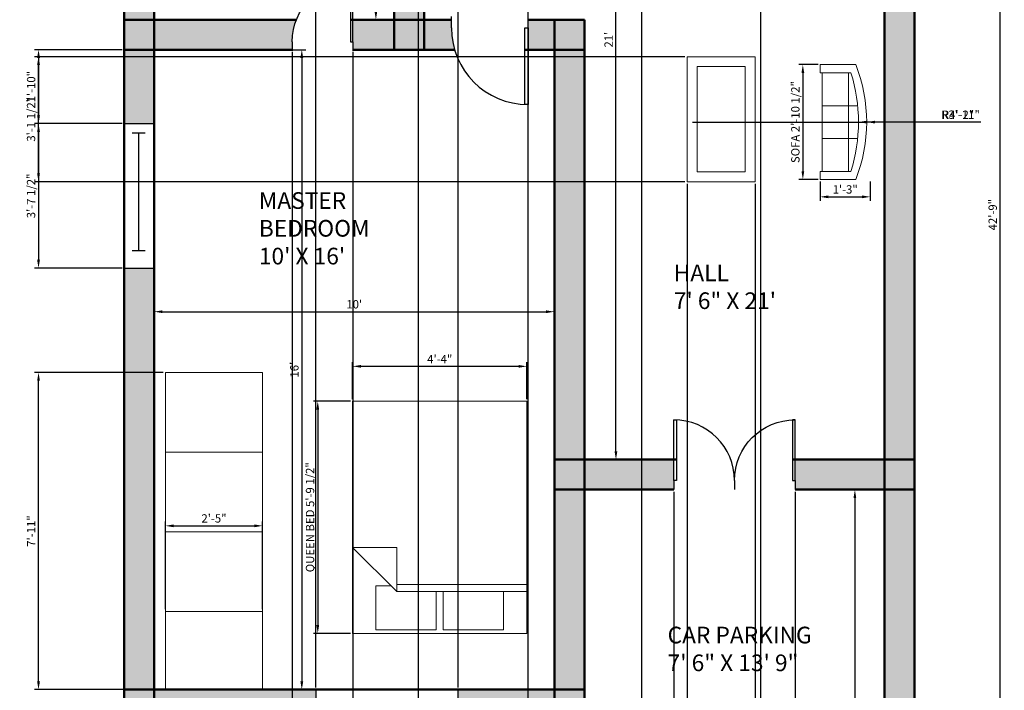
# Model space of a CAD drawing. Units: millimetres. Extents: x 2877 to 3173, y 802 to 1374.
# Tile 2 of 5: x 2877 to 3173, y 943 to 1144. Entities that reach past the tile are written whole.
import ezdxf

# ---------------------------------------------------------------- set-up
doc = ezdxf.new("R2010")
doc.units = ezdxf.units.MM
for name, color, linetype, lineweight in [('A-AREA-IDEN', 150, 'Continuous', 25), ('A-WALL-PATT', 3, 'Continuous', 13), ('dimensions', 140, 'Continuous', 18), ('doors', 10, 'Continuous', 25), ('furniture', 70, 'Continuous', 18), ('walls', 50, 'Continuous', 50), ('windows', 190, 'Continuous', 25)]:
    doc.layers.add(name, color=color, linetype=linetype, lineweight=lineweight)
doc.styles.get("Standard").update_dxf_attribs({"font": 'arial.ttf'})
doc.dimstyles.new('ISO-25', dxfattribs={"dimtxt": 2.5, "dimasz": 2.5, "dimexe": 1.25, "dimexo": 0.625, "dimtad": 1, "dimdec": 0, "dimlunit": 3, "dimtxsty": 'Standard', "dimcen": 2.5, "dimadec": 0, "dimazin": 0, "dimtfac": 1, "dimtdec": 0, "dimtmove": 0, "dimatfit": 3, "dimfxl": 1, "dimarcsym": 0})

# ---------------------------------------------------------------- blocks, each defined once
blk = doc.blocks.new('*U2')
for p, q in [((0, 0), (0, -6)), ((40, 0), (40, -6))]:
    blk.add_line(p, q)
blk.add_lwpolyline([(0, 0), (0, 40), (1.75, 40), (1.75, 0)], close=True)
blk.add_arc((0, 0), 40, 0, 90)
blk = doc.blocks.new('*U4')
for p, q in [((0, 4), (0, 0)), ((36, 4), (36, 0)), ((0, 2), (36, 2))]:
    blk.add_line(p, q)
blk = doc.blocks.new('Bed - Queen')
for p, q in [((0, -80.00003), (0, 0)), ((0, 0), (59.99999, 0)), ((59.99999, 0), (59.99999, -80.00003)), ((7.99999, -1.2), (28.79998, -1.2)), ((7.99999, -14.4), (7.99999, -1.2)), ((28.79998, -1.2), (28.79998, -14.4)), ((31.19999, -1.2), (51.99999, -1.2)), ((31.19999, -14.4), (31.19999, -1.2)), ((51.99999, -1.2), (51.99999, -16.4)), ((0, -14.4), (44.8, -14.4)), ((44.8, -16.8), (0, -16.8)), ((59.99999, -29.6), (44.8, -14.4)), ((44.8, -14.4), (44.8, -29.6)), ((51.99999, -16.4), (46.79936, -16.4)), ((44.8, -29.6), (59.99999, -29.6)), ((59.99999, -80.00003), (0, -80.00003))]:
    blk.add_line(p, q)
blk = doc.blocks.new('Sofa - Roundback 7 ft.')
for p, q in [((-12.00002, -32.4421), (-12.00003, -6.5971)), ((11.99997, -32.4421), (11.99998, -6.5971)), ((-36.000027, -34), (-36.000027, -11.4696)), ((-35.999844, -13.3819), (35.9998, -13.3819)), ((35.99998, -34), (35.99998, -11.4696)), ((-36.000027, -32.4421), (35.99998, -32.4421))]:
    blk.add_line(p, q)
for points in [[(-36.000027, -34), (-42.000027, -34), (-42.000027, -8)], [(41.99998, -8), (41.99998, -34), (35.99998, -34)]]:
    blk.add_lwpolyline(points)
for centre, radius, start, end in [((0, -114.25), 114.25, 68.43141, 111.5686), ((-0.00001, -127.1968), 121.1968, 72.72033, 107.2797)]:
    blk.add_arc(centre, radius, start, end)
blk = doc.blocks.new('*D15')
at = {"layer": 'Defpoints', "color": 0, "transparency": 16777216}
for p in [(3056.09, 1264.28), (3061, 1264.28), (3061, 1012.28)]:
    blk.add_point(p, dxfattribs=at)
at = {"layer": 'dimensions', "color": 0, "lineweight": -2, "transparency": 16777216}
for p, q in [((3060.38, 1264.28), (3054.84, 1264.28)), ((3056.09, 1014.78), (3056.09, 1261.78)), ((3060.38, 1012.28), (3054.84, 1012.28))]:
    blk.add_line(p, q, dxfattribs=at)
at = {"layer": 'dimensions', "color": 0, "transparency": 16777216}
for points in [[(3055.67, 1261.78), (3056.5, 1261.78), (3056.09, 1264.28)], [(3055.67, 1014.78), (3056.5, 1014.78), (3056.09, 1012.28)]]:
    blk.add_solid(points, dxfattribs=at)
at = {"layer": 'dimensions', "color": 0, "transparency": 16777216, "insert": (3054.21, 1138.28), "char_height": 2.5, "attachment_point": 5, "rotation": 90}
blk.add_mtext("21'", dxfattribs=at)
blk = doc.blocks.new('*D16')
at = {"layer": 'Defpoints', "color": 0, "transparency": 16777216}
for p in [(2984.11, 1204.28), (2984.11, 1144.28), (2984.11, 1144.28)]:
    blk.add_point(p, dxfattribs=at)
at = {"layer": 'dimensions', "color": 0, "lineweight": -2, "transparency": 16777216}
for p, q in [((2984.11, 1201.78), (2984.11, 1146.78)), ((2984.74, 1204.28), (2985.36, 1204.28)), ((2984.74, 1144.28), (2985.36, 1144.28))]:
    blk.add_line(p, q, dxfattribs=at)
at = {"layer": 'dimensions', "color": 0, "transparency": 16777216}
for points in [[(2983.69, 1201.78), (2984.53, 1201.78), (2984.11, 1204.28)], [(2983.69, 1146.78), (2984.53, 1146.78), (2984.11, 1144.28)]]:
    blk.add_solid(points, dxfattribs=at)
at = {"layer": 'dimensions', "color": 0, "transparency": 16777216, "insert": (2982.21, 1174.28), "char_height": 2.5, "attachment_point": 5, "rotation": 90}
blk.add_mtext("5'", dxfattribs=at)
blk = doc.blocks.new('*D18')
at = {"layer": 'Defpoints', "color": 0, "transparency": 16777216}
for p in [(2917.62, 1056.67), (3037.62, 1056.67), (3037.62, 1056.67)]:
    blk.add_point(p, dxfattribs=at)
at = {"layer": 'dimensions', "color": 0, "lineweight": -2, "transparency": 16777216}
for p, q in [((2917.62, 1057.29), (2917.62, 1057.92)), ((3037.62, 1057.29), (3037.62, 1057.92)), ((2920.12, 1056.67), (3035.12, 1056.67))]:
    blk.add_line(p, q, dxfattribs=at)
at = {"layer": 'dimensions', "color": 0, "transparency": 16777216}
for points in [[(2920.12, 1057.08), (2920.12, 1056.25), (2917.62, 1056.67)], [(3035.12, 1057.08), (3035.12, 1056.25), (3037.62, 1056.67)]]:
    blk.add_solid(points, dxfattribs=at)
at = {"layer": 'dimensions', "color": 0, "transparency": 16777216, "insert": (2977.62, 1058.57), "char_height": 2.5, "attachment_point": 5}
blk.add_mtext("10'", dxfattribs=at)
blk = doc.blocks.new('*D19')
at = {"layer": 'Defpoints', "color": 0, "transparency": 16777216}
for p in [(2948.77, 1135.28), (2950.14, 943.28), (2961.9, 943.28)]:
    blk.add_point(p, dxfattribs=at)
at = {"layer": 'dimensions', "color": 0, "lineweight": -2, "transparency": 16777216}
for p, q in [((2949.39, 1135.28), (2963.15, 1135.28)), ((2961.9, 1132.78), (2961.9, 945.78)), ((2950.76, 943.28), (2963.15, 943.28))]:
    blk.add_line(p, q, dxfattribs=at)
at = {"layer": 'dimensions', "color": 0, "transparency": 16777216}
for points in [[(2961.48, 1132.78), (2962.32, 1132.78), (2961.9, 1135.28)], [(2961.48, 945.78), (2962.32, 945.78), (2961.9, 943.28)]]:
    blk.add_solid(points, dxfattribs=at)
at = {"layer": 'dimensions', "color": 0, "transparency": 16777216, "insert": (2960, 1039.28), "char_height": 2.5, "attachment_point": 5, "rotation": 90}
blk.add_mtext("16'", dxfattribs=at)
blk = doc.blocks.new('*D20')
at = {"layer": 'Defpoints', "color": 0, "transparency": 16777216}
for p in [(3127.73, 1003.28), (3127.73, 838.28), (3127.73, 838.28)]:
    blk.add_point(p, dxfattribs=at)
at = {"layer": 'dimensions', "color": 0, "lineweight": -2, "transparency": 16777216}
for p, q in [((3128.35, 1003.28), (3128.98, 1003.28)), ((3127.73, 1000.78), (3127.73, 840.78)), ((3128.35, 838.28), (3128.98, 838.28))]:
    blk.add_line(p, q, dxfattribs=at)
at = {"layer": 'dimensions', "color": 0, "transparency": 16777216}
for points in [[(3127.31, 1000.78), (3128.14, 1000.78), (3127.73, 1003.28)], [(3127.31, 840.78), (3128.14, 840.78), (3127.73, 838.28)]]:
    blk.add_solid(points, dxfattribs=at)
at = {"layer": 'dimensions', "color": 0, "transparency": 16777216, "insert": (3125.83, 920.78), "char_height": 2.5, "attachment_point": 5, "rotation": 90}
blk.add_mtext('13\'-9"', dxfattribs=at)
blk = doc.blocks.new('*D28')
at = {"layer": 'Defpoints', "color": 0, "transparency": 16777216}
for p in [(2977.14, 1029.82), (2966.69, 960.17), (2977.14, 960.17)]:
    blk.add_point(p, dxfattribs=at)
at = {"layer": 'dimensions', "color": 0, "lineweight": -2, "transparency": 16777216}
for p, q in [((2976.51, 1029.82), (2965.44, 1029.82)), ((2966.69, 1027.32), (2966.69, 962.67)), ((2976.51, 960.17), (2965.44, 960.17))]:
    blk.add_line(p, q, dxfattribs=at)
at = {"layer": 'dimensions', "color": 0, "transparency": 16777216}
for points in [[(2966.27, 1027.32), (2967.1, 1027.32), (2966.69, 1029.82)], [(2966.27, 962.67), (2967.1, 962.67), (2966.69, 960.17)]]:
    blk.add_solid(points, dxfattribs=at)
at = {"layer": 'dimensions', "color": 0, "transparency": 16777216, "insert": (2964.69, 995), "char_height": 2.5, "attachment_point": 5, "rotation": 90}
blk.add_mtext('QUEEN BED 5\'-9 1/2"', dxfattribs=at)
blk = doc.blocks.new('*D29')
at = {"layer": 'Defpoints', "color": 0, "transparency": 16777216}
for p in [(2977.14, 1040.27), (2977.14, 1029.82), (3029.38, 1029.82)]:
    blk.add_point(p, dxfattribs=at)
at = {"layer": 'dimensions', "color": 0, "lineweight": -2, "transparency": 16777216}
for p, q in [((2977.14, 1030.45), (2977.14, 1041.52)), ((3026.88, 1040.27), (2979.64, 1040.27)), ((3029.38, 1030.45), (3029.38, 1041.52))]:
    blk.add_line(p, q, dxfattribs=at)
at = {"layer": 'dimensions', "color": 0, "transparency": 16777216}
for points in [[(2979.64, 1040.69), (2979.64, 1039.86), (2977.14, 1040.27)], [(3026.88, 1040.69), (3026.88, 1039.86), (3029.38, 1040.27)]]:
    blk.add_solid(points, dxfattribs=at)
at = {"layer": 'dimensions', "color": 0, "transparency": 16777216, "insert": (3003.26, 1042.15), "char_height": 2.5, "attachment_point": 5}
blk.add_mtext('4\'-4"', dxfattribs=at)
blk = doc.blocks.new('*D30')
at = {"layer": 'Defpoints', "color": 0, "transparency": 16777216}
for p in [(3117.31, 1130.79), (3112.13, 1096.3), (3117.31, 1096.3)]:
    blk.add_point(p, dxfattribs=at)
at = {"layer": 'dimensions', "color": 0, "lineweight": -2, "transparency": 16777216}
for p, q in [((3116.68, 1130.79), (3110.88, 1130.79)), ((3112.13, 1128.29), (3112.13, 1098.8)), ((3116.68, 1096.3), (3110.88, 1096.3))]:
    blk.add_line(p, q, dxfattribs=at)
at = {"layer": 'dimensions', "color": 0, "transparency": 16777216}
for points in [[(3111.72, 1128.29), (3112.55, 1128.29), (3112.13, 1130.79)], [(3111.72, 1098.8), (3112.55, 1098.8), (3112.13, 1096.3)]]:
    blk.add_solid(points, dxfattribs=at)
at = {"layer": 'dimensions', "color": 0, "transparency": 16777216, "insert": (3110.21, 1113.55), "char_height": 2.5, "attachment_point": 5, "rotation": 90}
blk.add_mtext('SOFA 2\'-10 1/2"', dxfattribs=at)
blk = doc.blocks.new('*D31')
at = {"layer": 'Defpoints', "color": 0, "transparency": 16777216}
for p in [(3117.31, 1096.3), (3132.36, 1096.3), (3132.36, 1091.13)]:
    blk.add_point(p, dxfattribs=at)
at = {"layer": 'dimensions', "color": 0, "lineweight": -2, "transparency": 16777216}
for p, q in [((3117.31, 1095.68), (3117.31, 1089.88)), ((3132.36, 1095.68), (3132.36, 1089.88)), ((3119.81, 1091.13), (3129.86, 1091.13))]:
    blk.add_line(p, q, dxfattribs=at)
at = {"layer": 'dimensions', "color": 0, "transparency": 16777216}
for points in [[(3119.81, 1091.55), (3119.81, 1090.71), (3117.31, 1091.13)], [(3129.86, 1091.55), (3129.86, 1090.71), (3132.36, 1091.13)]]:
    blk.add_solid(points, dxfattribs=at)
at = {"layer": 'dimensions', "color": 0, "transparency": 16777216, "insert": (3124.83, 1093.03), "char_height": 2.5, "attachment_point": 5}
blk.add_mtext('1\'-3"', dxfattribs=at)
blk = doc.blocks.new('*D35')
at = {"layer": 'Defpoints', "color": 0, "transparency": 16777216}
for p in [(3145.62, 1342.28), (3171.28, 1342.28), (3145.62, 829.28)]:
    blk.add_point(p, dxfattribs=at)
at = {"layer": 'dimensions', "color": 0, "lineweight": -2, "transparency": 16777216}
for p, q in [((3146.25, 1342.28), (3172.53, 1342.28)), ((3171.28, 831.78), (3171.28, 1339.78)), ((3146.25, 829.28), (3172.53, 829.28))]:
    blk.add_line(p, q, dxfattribs=at)
at = {"layer": 'dimensions', "color": 0, "transparency": 16777216}
for points in [[(3170.87, 1339.78), (3171.7, 1339.78), (3171.28, 1342.28)], [(3170.87, 831.78), (3171.7, 831.78), (3171.28, 829.28)]]:
    blk.add_solid(points, dxfattribs=at)
at = {"layer": 'dimensions', "color": 0, "transparency": 16777216, "insert": (3169.38, 1085.78), "char_height": 2.5, "attachment_point": 5, "rotation": 90}
blk.add_mtext('42\'-9"', dxfattribs=at)
blk = doc.blocks.new('*D36')
at = {"layer": 'Defpoints', "color": 0, "transparency": 16777216}
for p in [(2908.62, 1301.43), (2917.62, 1301.43), (2917.62, 803.61)]:
    blk.add_point(p, dxfattribs=at)
at = {"layer": 'dimensions', "color": 0, "lineweight": -2, "transparency": 16777216}
for p, q in [((2908.62, 1300.81), (2908.62, 802.36)), ((2917.62, 1300.81), (2917.62, 802.36)), ((2911.12, 803.61), (2915.12, 803.61))]:
    blk.add_line(p, q, dxfattribs=at)
at = {"layer": 'dimensions', "color": 0, "transparency": 16777216}
for points in [[(2911.12, 804.03), (2911.12, 803.2), (2908.62, 803.61)], [(2915.12, 804.03), (2915.12, 803.2), (2917.62, 803.61)]]:
    blk.add_solid(points, dxfattribs=at)
at = {"layer": 'dimensions', "color": 0, "transparency": 16777216, "insert": (2913.12, 805.52), "char_height": 2.5, "attachment_point": 5}
blk.add_mtext('0\'-9"', dxfattribs=at)
blk = doc.blocks.new('*D40')
at = {"layer": 'Defpoints', "color": 0, "transparency": 16777216}
for p in [(3063.76, 1264.28), (3099.39, 1264.17), (3099.39, 803.61)]:
    blk.add_point(p, dxfattribs=at)
at = {"layer": 'dimensions', "color": 0, "lineweight": -2, "transparency": 16777216}
for p, q in [((3063.76, 1263.65), (3063.76, 802.36)), ((3099.39, 1263.55), (3099.39, 802.36)), ((3066.26, 803.61), (3096.89, 803.61))]:
    blk.add_line(p, q, dxfattribs=at)
at = {"layer": 'dimensions', "color": 0, "transparency": 16777216}
for points in [[(3066.26, 804.03), (3066.26, 803.2), (3063.76, 803.61)], [(3096.89, 804.03), (3096.89, 803.2), (3099.39, 803.61)]]:
    blk.add_solid(points, dxfattribs=at)
at = {"layer": 'dimensions', "color": 0, "transparency": 16777216, "insert": (3081.57, 805.53), "char_height": 2.5, "attachment_point": 5}
blk.add_mtext('2\'-11 1/2"', dxfattribs=at)
blk = doc.blocks.new('*D42')
at = {"layer": 'Defpoints', "color": 0, "transparency": 16777216}
for p in [(3073.41, 1003.28), (3109.83, 1003.28), (3109.83, 803.61)]:
    blk.add_point(p, dxfattribs=at)
at = {"layer": 'dimensions', "color": 0, "lineweight": -2, "transparency": 16777216}
for p, q in [((3073.41, 1002.65), (3073.41, 802.36)), ((3109.83, 1002.65), (3109.83, 802.36)), ((3075.91, 803.61), (3107.33, 803.61))]:
    blk.add_line(p, q, dxfattribs=at)
at = {"layer": 'dimensions', "color": 0, "transparency": 16777216}
for points in [[(3075.91, 804.03), (3075.91, 803.2), (3073.41, 803.61)], [(3107.33, 804.03), (3107.33, 803.2), (3109.83, 803.61)]]:
    blk.add_solid(points, dxfattribs=at)
at = {"layer": 'dimensions', "color": 0, "transparency": 16777216, "insert": (3091.62, 805.53), "char_height": 2.5, "attachment_point": 5}
blk.add_mtext('3\'-0 1/2"', dxfattribs=at)
blk = doc.blocks.new('*D43')
at = {"layer": 'Defpoints', "color": 0, "transparency": 16777216}
for p in [(3037.62, 1003.28), (3073.41, 1003.28), (3073.41, 803.61)]:
    blk.add_point(p, dxfattribs=at)
at = {"layer": 'dimensions', "color": 0, "lineweight": -2, "transparency": 16777216}
for p, q in [((3037.62, 1002.65), (3037.62, 802.36)), ((3073.41, 1002.65), (3073.41, 802.36)), ((3040.12, 803.61), (3070.91, 803.61))]:
    blk.add_line(p, q, dxfattribs=at)
at = {"layer": 'dimensions', "color": 0, "transparency": 16777216}
for points in [[(3040.12, 804.03), (3040.12, 803.2), (3037.62, 803.61)], [(3070.91, 804.03), (3070.91, 803.2), (3073.41, 803.61)]]:
    blk.add_solid(points, dxfattribs=at)
at = {"layer": 'dimensions', "color": 0, "transparency": 16777216, "insert": (3055.52, 805.52), "char_height": 2.5, "attachment_point": 5}
blk.add_mtext('3\'-0"', dxfattribs=at)
blk = doc.blocks.new('*D44')
at = {"layer": 'Defpoints', "color": 0, "transparency": 16777216}
for p in [(2996.81, 1237.82), (3029.69, 1237.82), (3029.69, 803.61)]:
    blk.add_point(p, dxfattribs=at)
at = {"layer": 'dimensions', "color": 0, "lineweight": -2, "transparency": 16777216}
for p, q in [((2996.81, 1237.19), (2996.81, 802.36)), ((3029.69, 1237.19), (3029.69, 802.36)), ((2999.31, 803.61), (3027.19, 803.61))]:
    blk.add_line(p, q, dxfattribs=at)
at = {"layer": 'dimensions', "color": 0, "transparency": 16777216}
for points in [[(2999.31, 804.03), (2999.31, 803.2), (2996.81, 803.61)], [(3027.19, 804.03), (3027.19, 803.2), (3029.69, 803.61)]]:
    blk.add_solid(points, dxfattribs=at)
at = {"layer": 'dimensions', "color": 0, "transparency": 16777216, "insert": (3013.25, 805.52), "char_height": 2.5, "attachment_point": 5}
blk.add_mtext('2\'-9"', dxfattribs=at)
blk = doc.blocks.new('*D46')
at = {"layer": 'Defpoints', "color": 0, "transparency": 16777216}
for p in [(2959.04, 1135.28), (2977.25, 1135.28), (2977.25, 803.61)]:
    blk.add_point(p, dxfattribs=at)
at = {"layer": 'dimensions', "color": 0, "lineweight": -2, "transparency": 16777216}
for p, q in [((2959.04, 1134.65), (2959.04, 802.36)), ((2977.25, 1134.65), (2977.25, 802.36)), ((2961.54, 803.61), (2974.75, 803.61))]:
    blk.add_line(p, q, dxfattribs=at)
at = {"layer": 'dimensions', "color": 0, "transparency": 16777216}
for points in [[(2961.54, 804.03), (2961.54, 803.2), (2959.04, 803.61)], [(2974.75, 804.03), (2974.75, 803.2), (2977.25, 803.61)]]:
    blk.add_solid(points, dxfattribs=at)
at = {"layer": 'dimensions', "color": 0, "transparency": 16777216, "insert": (2968.15, 805.52), "char_height": 2.5, "attachment_point": 5}
blk.add_mtext('1\'-6"', dxfattribs=at)
blk = doc.blocks.new('*D47')
at = {"layer": 'Defpoints', "color": 0, "transparency": 16777216}
for p in [(2908.62, 1135.28), (2959.04, 1135.28), (2959.04, 803.61)]:
    blk.add_point(p, dxfattribs=at)
at = {"layer": 'dimensions', "color": 0, "lineweight": -2, "transparency": 16777216}
for p, q in [((2908.62, 1134.65), (2908.62, 802.36)), ((2959.04, 1134.65), (2959.04, 802.36)), ((2911.12, 803.61), (2956.54, 803.61))]:
    blk.add_line(p, q, dxfattribs=at)
at = {"layer": 'dimensions', "color": 0, "transparency": 16777216}
for points in [[(2911.12, 804.03), (2911.12, 803.2), (2908.62, 803.61)], [(2956.54, 804.03), (2956.54, 803.2), (2959.04, 803.61)]]:
    blk.add_solid(points, dxfattribs=at)
at = {"layer": 'dimensions', "color": 0, "transparency": 16777216, "insert": (2933.83, 805.53), "char_height": 2.5, "attachment_point": 5}
blk.add_mtext('4\'-2 1/2"', dxfattribs=at)
blk = doc.blocks.new('*D56')
at = {"layer": 'Defpoints', "color": 0, "transparency": 16777216}
for p in [(2908.62, 1135.28), (2882.96, 1113.08), (2908.62, 1113.08)]:
    blk.add_point(p, dxfattribs=at)
at = {"layer": 'dimensions', "color": 0, "lineweight": -2, "transparency": 16777216}
for p, q in [((2908, 1135.28), (2881.71, 1135.28)), ((2882.96, 1132.78), (2882.96, 1115.58)), ((2908, 1113.08), (2881.71, 1113.08))]:
    blk.add_line(p, q, dxfattribs=at)
at = {"layer": 'dimensions', "color": 0, "transparency": 16777216}
for points in [[(2882.54, 1132.78), (2883.38, 1132.78), (2882.96, 1135.28)], [(2882.54, 1115.58), (2883.38, 1115.58), (2882.96, 1113.08)]]:
    blk.add_solid(points, dxfattribs=at)
at = {"layer": 'dimensions', "color": 0, "transparency": 16777216, "insert": (2881.06, 1124.18), "char_height": 2.5, "attachment_point": 5, "rotation": 90}
blk.add_mtext('1\'-10"', dxfattribs=at)
blk = doc.blocks.new('*D57')
at = {"layer": 'Defpoints', "color": 0, "transparency": 16777216}
for p in [(2908.62, 1113.08), (2882.96, 1069.77), (2908.62, 1069.77)]:
    blk.add_point(p, dxfattribs=at)
at = {"layer": 'dimensions', "color": 0, "lineweight": -2, "transparency": 16777216}
for p, q in [((2908, 1113.08), (2881.71, 1113.08)), ((2882.96, 1110.58), (2882.96, 1072.27)), ((2908, 1069.77), (2881.71, 1069.77))]:
    blk.add_line(p, q, dxfattribs=at)
at = {"layer": 'dimensions', "color": 0, "transparency": 16777216}
for points in [[(2882.54, 1110.58), (2883.38, 1110.58), (2882.96, 1113.08)], [(2882.54, 1072.27), (2883.38, 1072.27), (2882.96, 1069.77)]]:
    blk.add_solid(points, dxfattribs=at)
at = {"layer": 'dimensions', "color": 0, "transparency": 16777216, "insert": (2881.04, 1091.42), "char_height": 2.5, "attachment_point": 5, "rotation": 90}
blk.add_mtext('3\'-7 1/2"', dxfattribs=at)
blk = doc.blocks.new('*D58')
at = {"layer": 'Defpoints', "color": 0, "transparency": 16777216}
for p in [(2966.07, 1367.94), (2908.62, 943.28), (2966.07, 943.28)]:
    blk.add_point(p, dxfattribs=at)
at = {"layer": 'dimensions', "color": 0, "lineweight": -2, "transparency": 16777216}
for p, q in [((2908.62, 943.9), (2908.62, 1369.19)), ((2911.12, 1367.94), (2963.57, 1367.94)), ((2966.07, 943.9), (2966.07, 1369.19))]:
    blk.add_line(p, q, dxfattribs=at)
at = {"layer": 'dimensions', "color": 0, "transparency": 16777216}
for points in [[(2911.12, 1368.36), (2911.12, 1367.52), (2908.62, 1367.94)], [(2963.57, 1368.36), (2963.57, 1367.52), (2966.07, 1367.94)]]:
    blk.add_solid(points, dxfattribs=at)
at = {"layer": 'dimensions', "color": 0, "transparency": 16777216, "insert": (2937.34, 1369.86), "char_height": 2.5, "attachment_point": 5}
blk.add_mtext('4\'-9 1/2"', dxfattribs=at)
blk = doc.blocks.new('*D59')
at = {"layer": 'Defpoints', "color": 0, "transparency": 16777216}
for p in [(3008.74, 1367.94), (2966.07, 943.28), (3008.74, 943.28)]:
    blk.add_point(p, dxfattribs=at)
at = {"layer": 'dimensions', "color": 0, "lineweight": -2, "transparency": 16777216}
for p, q in [((2966.07, 943.9), (2966.07, 1369.19)), ((2968.57, 1367.94), (3006.24, 1367.94)), ((3008.74, 943.9), (3008.74, 1369.19))]:
    blk.add_line(p, q, dxfattribs=at)
at = {"layer": 'dimensions', "color": 0, "transparency": 16777216}
for points in [[(2968.57, 1368.36), (2968.57, 1367.52), (2966.07, 1367.94)], [(3006.24, 1368.36), (3006.24, 1367.52), (3008.74, 1367.94)]]:
    blk.add_solid(points, dxfattribs=at)
at = {"layer": 'dimensions', "color": 0, "transparency": 16777216, "insert": (2987.4, 1369.86), "char_height": 2.5, "attachment_point": 5}
blk.add_mtext('3\'-6 1/2"', dxfattribs=at)
blk = doc.blocks.new('*D62')
at = {"layer": 'Defpoints', "color": 0, "transparency": 16777216}
for p in [(2950.14, 992.43), (2921, 966.77), (2950.14, 966.77)]:
    blk.add_point(p, dxfattribs=at)
at = {"layer": 'dimensions', "color": 0, "lineweight": -2, "transparency": 16777216}
for p, q in [((2921, 967.39), (2921, 993.68)), ((2923.5, 992.43), (2947.64, 992.43)), ((2950.14, 967.39), (2950.14, 993.68))]:
    blk.add_line(p, q, dxfattribs=at)
at = {"layer": 'dimensions', "color": 0, "transparency": 16777216}
for points in [[(2923.5, 992.85), (2923.5, 992.01), (2921, 992.43)], [(2947.64, 992.85), (2947.64, 992.01), (2950.14, 992.43)]]:
    blk.add_solid(points, dxfattribs=at)
at = {"layer": 'dimensions', "color": 0, "transparency": 16777216, "insert": (2935.57, 994.33), "char_height": 2.5, "attachment_point": 5}
blk.add_mtext('2\'-5"', dxfattribs=at)
blk = doc.blocks.new('*D63')
at = {"layer": 'Defpoints', "color": 0, "transparency": 16777216}
for p in [(2882.96, 1038.44), (2921, 1038.44), (2921, 943.28)]:
    blk.add_point(p, dxfattribs=at)
at = {"layer": 'dimensions', "color": 0, "lineweight": -2, "transparency": 16777216}
for p, q in [((2920.38, 1038.44), (2881.71, 1038.44)), ((2882.96, 945.78), (2882.96, 1035.94)), ((2920.38, 943.28), (2881.71, 943.28))]:
    blk.add_line(p, q, dxfattribs=at)
at = {"layer": 'dimensions', "color": 0, "transparency": 16777216}
for points in [[(2882.54, 1035.94), (2883.38, 1035.94), (2882.96, 1038.44)], [(2882.54, 945.78), (2883.38, 945.78), (2882.96, 943.28)]]:
    blk.add_solid(points, dxfattribs=at)
at = {"layer": 'dimensions', "color": 0, "transparency": 16777216, "insert": (2881.08, 990.86), "char_height": 2.5, "attachment_point": 5, "rotation": 90}
blk.add_mtext('7\'-11"', dxfattribs=at)
blk = doc.blocks.new('*D64')
at = {"layer": 'Defpoints', "color": 0, "transparency": 16777216}
for p in [(3077.4, 1095.65), (3097.88, 1095.65), (3097.88, 803.61)]:
    blk.add_point(p, dxfattribs=at)
at = {"layer": 'dimensions', "color": 0, "lineweight": -2, "transparency": 16777216}
for p, q in [((3077.4, 1095.02), (3077.4, 802.36)), ((3097.88, 1095.02), (3097.88, 802.36)), ((3079.9, 803.61), (3095.38, 803.61))]:
    blk.add_line(p, q, dxfattribs=at)
at = {"layer": 'dimensions', "color": 0, "transparency": 16777216}
for points in [[(3079.9, 804.03), (3079.9, 803.2), (3077.4, 803.61)], [(3095.38, 804.03), (3095.38, 803.2), (3097.88, 803.61)]]:
    blk.add_solid(points, dxfattribs=at)
at = {"layer": 'dimensions', "color": 0, "transparency": 16777216, "insert": (3087.64, 805.53), "char_height": 2.5, "attachment_point": 5}
blk.add_mtext('1\'-8 1/2"', dxfattribs=at)
blk = doc.blocks.new('*D65')
at = {"layer": 'Defpoints', "color": 0, "transparency": 16777216}
for p in [(2882.96, 1133.18), (3077.4, 1133.18), (3077.4, 1095.65)]:
    blk.add_point(p, dxfattribs=at)
at = {"layer": 'dimensions', "color": 0, "lineweight": -2, "transparency": 16777216}
for p, q in [((3076.77, 1133.18), (2881.71, 1133.18)), ((2882.96, 1098.15), (2882.96, 1130.68)), ((3076.77, 1095.65), (2881.71, 1095.65))]:
    blk.add_line(p, q, dxfattribs=at)
at = {"layer": 'dimensions', "color": 0, "transparency": 16777216}
for points in [[(2882.54, 1130.68), (2883.38, 1130.68), (2882.96, 1133.18)], [(2882.54, 1098.15), (2883.38, 1098.15), (2882.96, 1095.65)]]:
    blk.add_solid(points, dxfattribs=at)
at = {"layer": 'dimensions', "color": 0, "transparency": 16777216, "insert": (2881.04, 1114.41), "char_height": 2.5, "attachment_point": 5, "rotation": 90}
blk.add_mtext('3\'-1 1/2"', dxfattribs=at)
blk = doc.blocks.new('*D66')
at = {"layer": 'Defpoints', "color": 0, "transparency": 16777216}
for p in [(2917.62, 1257.52), (2996.81, 1237.82), (2996.81, 803.61)]:
    blk.add_point(p, dxfattribs=at)
at = {"layer": 'dimensions', "color": 0, "lineweight": -2, "transparency": 16777216}
for p, q in [((2917.62, 1256.89), (2917.62, 802.36)), ((2996.81, 1237.19), (2996.81, 802.36)), ((2920.12, 803.61), (2994.31, 803.61))]:
    blk.add_line(p, q, dxfattribs=at)
at = {"layer": 'dimensions', "color": 0, "transparency": 16777216}
for points in [[(2920.12, 804.03), (2920.12, 803.2), (2917.62, 803.61)], [(2994.31, 804.03), (2994.31, 803.2), (2996.81, 803.61)]]:
    blk.add_solid(points, dxfattribs=at)
at = {"layer": 'dimensions', "color": 0, "transparency": 16777216, "insert": (2957.22, 805.52), "char_height": 2.5, "attachment_point": 5}
blk.add_mtext('6\'-7"', dxfattribs=at)
blk = doc.blocks.new('*D75')
at = {"layer": 'Defpoints', "color": 0, "transparency": 16777216}
for p in [(3079.04, 1113.55), (3128.8, 1113.55)]:
    blk.add_point(p, dxfattribs=at)
at = {"layer": 'dimensions', "color": 0, "lineweight": -2, "transparency": 16777216}
for p, q in [((3079.04, 1113.55), (3128.8, 1113.55)), ((3163.81, 1113.55), (3131.3, 1113.55))]:
    blk.add_line(p, q, dxfattribs=at)
at = {"layer": 'dimensions', "color": 0, "transparency": 16777216}
blk.add_solid([(3131.3, 1113.97), (3131.3, 1113.13), (3128.8, 1113.55)], dxfattribs=at)
at = {"layer": 'dimensions', "color": 0, "transparency": 16777216, "insert": (3158.66, 1115.43), "char_height": 2.5, "attachment_point": 5, "rotation": 0.0001}
blk.add_mtext('R4\'-2"', dxfattribs=at)
blk = doc.blocks.new('*D76')
at = {"layer": 'Defpoints', "color": 0, "transparency": 16777216}
for p in [(3084.36, 1113.55), (3131.27, 1113.55)]:
    blk.add_point(p, dxfattribs=at)
at = {"layer": 'dimensions', "color": 0, "lineweight": -2, "transparency": 16777216}
for p, q in [((3084.36, 1113.55), (3131.27, 1113.55)), ((3165.53, 1113.55), (3133.77, 1113.55))]:
    blk.add_line(p, q, dxfattribs=at)
at = {"layer": 'dimensions', "color": 0, "transparency": 16777216}
blk.add_solid([(3133.77, 1113.97), (3133.77, 1113.13), (3131.27, 1113.55)], dxfattribs=at)
at = {"layer": 'dimensions', "color": 0, "transparency": 16777216, "insert": (3159.41, 1115.45), "char_height": 2.5, "attachment_point": 5, "rotation": 0.0001}
blk.add_mtext('R3\'-11"', dxfattribs=at)

msp = doc.modelspace()

# ---------------------------------------------------------------- hatches: boundary and pattern name
at = {"layer": 'A-WALL-PATT'}
h = msp.add_hatch(color=256, dxfattribs=at)
h.dxf.hatch_style = 1
h.paths.add_polyline_path([(3046.62, 1333.28), (3037.62, 1333.28), (3037.62, 1273.28), (3046.62, 1273.28)])
h.paths.add_polyline_path([(3046.62, 1273.28), (3037.62, 1273.28), (3037.62, 1264.28), (3046.62, 1264.28)])
h.paths.add_polyline_path([(3046.62, 1264.28), (3037.62, 1264.28), (3037.62, 1204.28), (3046.62, 1204.28)])
h.paths.add_polyline_path([(3136.62, 1273.28), (3099.39, 1273.28), (3099.39, 1264.28), (3136.62, 1264.28)])
h.paths.add_polyline_path([(3145.62, 1273.28), (3136.62, 1273.28), (3136.62, 1264.28), (3145.62, 1264.28)])
h.paths.add_polyline_path([(3145.62, 1264.28), (3136.62, 1264.28), (3136.62, 1198.76), (3145.62, 1198.76)])
h.paths.add_polyline_path([(3145.62, 1333.28), (3136.62, 1333.28), (3136.62, 1273.28), (3145.62, 1273.28)])
h.paths.add_polyline_path([(3145.62, 1342.28), (3136.62, 1342.28), (3136.62, 1333.28), (3145.62, 1333.28)])
h.paths.add_polyline_path([(3136.62, 1342.28), (3046.62, 1342.28), (3046.62, 1333.28), (3136.62, 1333.28)])
h.paths.add_polyline_path([(3046.62, 1342.28), (3037.62, 1342.28), (3037.62, 1333.28), (3046.62, 1333.28)])
h.paths.add_polyline_path([(2917.62, 1333.28), (2908.62, 1333.28), (2908.62, 1301.43), (2917.62, 1301.43)])
h.paths.add_polyline_path([(2917.62, 1257.52), (2908.62, 1257.52), (2908.62, 1213.28), (2917.62, 1213.28)])
h.paths.add_polyline_path([(2989.62, 1213.28), (2917.62, 1213.28), (2917.62, 1204.28), (2989.62, 1204.28)])
h.paths.add_polyline_path([(2998.62, 1213.28), (2989.62, 1213.28), (2989.62, 1204.28), (2998.62, 1204.28)])
h.paths.add_polyline_path([(2998.62, 1204.28), (2989.62, 1204.28), (2989.62, 1144.28), (2998.62, 1144.28)])
h.paths.add_polyline_path([(2998.62, 1144.28), (2989.62, 1144.28), (2989.62, 1135.28), (2998.62, 1135.28)])
h.paths.add_polyline_path([(2989.62, 1144.28), (2977.25, 1144.28), (2977.25, 1137.64), (2977.25, 1135.28), (2989.62, 1135.28)])
h.paths.add_polyline_path([(3006.77, 1141.79), (3006.77, 1144.28), (2998.62, 1144.28), (2998.62, 1135.28), (3007.71, 1135.28, -0.072018)])
h.paths.add_polyline_path([(3046.62, 1135.28), (3037.62, 1135.28), (3037.62, 1012.28), (3046.62, 1012.28)])
h.paths.add_polyline_path([(3046.62, 1144.28), (3037.62, 1144.28), (3037.62, 1135.28), (3046.62, 1135.28)])
h.paths.add_polyline_path([(3037.62, 1144.28), (3029.73, 1144.28), (3029.73, 1141.79), (3029.73, 1135.28), (3037.62, 1135.28)])
h.paths.add_polyline_path([(3145.62, 1158.87), (3136.62, 1158.87), (3136.62, 1012.28), (3145.62, 1012.28)])
h.paths.add_polyline_path([(3145.62, 1003.28), (3136.62, 1003.28), (3136.62, 838.28), (3145.62, 838.28)])
h.paths.add_polyline_path([(3145.62, 1012.28), (3136.62, 1012.28), (3136.62, 1003.28), (3145.62, 1003.28)])
h.paths.add_polyline_path([(3136.62, 1012.28), (3109.83, 1012.28), (3109.83, 1006.01), (3109.83, 1003.28), (3136.62, 1003.28)])
h.paths.add_polyline_path([(3073.41, 1012.28), (3046.62, 1012.28), (3046.62, 1003.28), (3073.41, 1003.28), (3073.41, 1006.01)])
h.paths.add_polyline_path([(3046.62, 1012.28), (3037.62, 1012.28), (3037.62, 1003.28), (3046.62, 1003.28)])
h.paths.add_polyline_path([(3046.62, 1003.28), (3037.62, 1003.28), (3037.62, 943.28), (3046.62, 943.28)])
h.paths.add_polyline_path([(3136.62, 838.28), (2917.62, 838.28), (2917.62, 829.28), (3136.62, 829.28)])
h.paths.add_polyline_path([(3145.62, 838.28), (3136.62, 838.28), (3136.62, 829.28), (3145.62, 829.28)])
h.paths.add_polyline_path([(2917.62, 934.28), (2908.62, 934.28), (2908.62, 838.28), (2917.62, 838.28)])
h.paths.add_polyline_path([(2917.62, 838.28), (2908.62, 838.28), (2908.62, 829.28), (2917.62, 829.28)])
h.paths.add_polyline_path([(2917.62, 943.28), (2908.62, 943.28), (2908.62, 934.28), (2917.62, 934.28)])
h.paths.add_polyline_path([(2966.07, 943.28), (2917.62, 943.28), (2917.62, 934.28), (2966.07, 934.28)])
h.paths.add_polyline_path([(3046.62, 943.28), (3037.62, 943.28), (3037.62, 934.28), (3046.62, 934.28)])
h.paths.add_polyline_path([(3037.62, 943.28), (3008.74, 943.28), (3008.74, 934.28), (3037.62, 934.28)])
h = msp.add_hatch(color=256, dxfattribs=at)
h.dxf.hatch_style = 1
h.paths.add_polyline_path([(2917.62, 1204.28), (2908.62, 1204.28), (2908.62, 1186.06), (2917.62, 1186.06)])
h.paths.add_polyline_path([(2917.62, 1156.99), (2908.62, 1156.99), (2908.62, 1144.28), (2917.62, 1144.28)])
h = msp.add_hatch(color=256, dxfattribs=at)
h.dxf.hatch_style = 1
h.paths.add_polyline_path([(2917.62, 1069.77), (2908.62, 1069.77), (2908.62, 943.28), (2917.62, 943.28)])
h.paths.add_polyline_path([(2917.62, 1144.28), (2908.62, 1144.28), (2908.62, 1135.28), (2917.62, 1135.28)])
h.paths.add_polyline_path([(2960.29, 1144.28), (2917.62, 1144.28), (2917.62, 1135.28), (2959.04, 1135.28), (2959.04, 1137.64, -0.093504)])
h.paths.add_polyline_path([(2917.62, 1135.28), (2908.62, 1135.28), (2908.62, 1113.08), (2917.62, 1113.08)])

# ---------------------------------------------------------------- linework, layer by layer
at = {"layer": 'furniture'}
for p, q in [((2921, 1038.44), (2950.14, 1038.44)), ((2921, 943.28), (2921, 1038.44)), ((2950.14, 1038.44), (2950.14, 943.28)), ((2921, 1014.55), (2950.14, 1014.55)), ((2921, 990.66), (2950.14, 990.66)), ((2921, 966.77), (2950.14, 966.77)), ((2950.14, 943.28), (2921, 943.28))]:
    msp.add_line(p, q, dxfattribs=at)
for points in [[(3077.4, 1133.18), (3097.88, 1133.18), (3097.88, 1095.65), (3077.4, 1095.65)], [(3080.4, 1130.18), (3094.88, 1130.18), (3094.88, 1098.65), (3080.4, 1098.65)]]:
    msp.add_lwpolyline(points, close=True, dxfattribs=at)
at = {"layer": 'walls'}
for p, q in [((2908.62, 1342.28), (2908.62, 829.28)), ((2917.62, 1342.28), (2917.62, 829.28)), ((3136.62, 1342.28), (3136.62, 829.28)), ((3145.62, 1342.28), (3145.62, 829.28)), ((2989.62, 1213.28), (2989.62, 1135.28)), ((2998.62, 1213.28), (2998.62, 1135.28)), ((2908.62, 1144.28), (2960.29, 1144.28)), ((2976.46, 1144.28), (3006.77, 1144.28)), ((3029.73, 1144.28), (3046.62, 1144.28)), ((3037.62, 1144.28), (3037.62, 934.28)), ((3046.62, 1144.28), (3046.62, 934.28)), ((2908.62, 1135.28), (2959.04, 1135.28)), ((2977.25, 1135.28), (3007.71, 1135.28)), ((3028.73, 1135.28), (3046.62, 1135.28)), ((3037.62, 1012.28), (3074.21, 1012.28)), ((3109.04, 1012.28), (3145.62, 1012.28)), ((3037.62, 1003.28), (3073.41, 1003.28)), ((3109.83, 1003.28), (3145.62, 1003.28)), ((2908.62, 943.28), (3046.62, 943.28))]:
    msp.add_line(p, q, dxfattribs=at)
at = {"layer": 'windows'}
for p, q in [((2908.62, 1113.08), (2917.62, 1113.08)), ((2908.62, 1069.77), (2917.62, 1069.77)), ((2966.07, 943.28), (2966.07, 934.28)), ((3008.74, 934.28), (3008.74, 943.28))]:
    msp.add_line(p, q, dxfattribs=at)

# ---------------------------------------------------------------- block references
at = {"layer": 'doors', "yscale": 0.4552510015893225, "zscale": 0.4552510015893225}
for p, xscale in [((2977.25, 1137.64), -0.4552510015893225), ((3073.41, 1006.01), 0.4552510015893225), ((3109.83, 1006.01), -0.4552510015893225)]:
    msp.add_blockref('*U2', p, dxfattribs=dict(at, xscale=xscale))
at = {"layer": 'doors', "xscale": 0.5739608518723968, "yscale": 0.5739608518723968, "zscale": 0.5739608518723968, "rotation": 180}
msp.add_blockref('*U2', (3029.73, 1141.79), dxfattribs=at)
at = {"layer": 'furniture'}
for name, p, xscale, yscale, zscale, rotation in [('Sofa - Roundback 7 ft.', (3131.27, 1113.55), 0.4106027653656436, 0.4106027653656436, 0.4106027653656436, 270), ('Bed - Queen', (3029.38, 960.17), 0.8707200715435497, 0.8707200715435497, 0.8707200715435497, 180)]:
    msp.add_blockref(name, p, dxfattribs=dict(at, xscale=xscale, yscale=yscale, zscale=zscale, rotation=rotation))
at = {"layer": 'windows', "xscale": 0.9804508946843826, "yscale": 0.9804508946843826, "zscale": 0.9804508946843826, "rotation": 90}
msp.add_blockref('*U4', (2914.98, 1075.06), dxfattribs=at)

# ---------------------------------------------------------------- texts
at = {"layer": 'A-AREA-IDEN', "char_height": 5, "attachment_point": 1}
for s, width, insert in [("MASTER\\PBEDROOM\\P10' X 16'", 71.9354, (2949.02, 1092.52)), ('HALL\\P7\' 6" X 21\'', 53.3551, (3073.43, 1070.8)), ('CAR PARKING\\P7\' 6" X 13\' 9"', 53.6382, (3071.58, 962.16))]:
    msp.add_mtext_dynamic_manual_height_columns(s, width=width, gutter_width=12.5, heights=[0], dxfattribs=dict(at, insert=insert))

# ---------------------------------------------------------------- dimensions: what is measured, and where the dimension line sits
at = {"layer": 'dimensions'}
for base, p1, p2, override, picture, middle in [((2966.066, 1367.9388), (2908.6223, 943.2763), (2966.066, 943.2763), {"dimdec": 1, "dimlfac": 1, "dimrnd": 0, "dimzin": 1, "dimdsep": 46, "dimlunit": 4, "dimfrac": 2}, '*D58', (2937.3441, 1369.8564)), ((3008.74, 1367.94), (2966.07, 943.28), (3008.74, 943.28), {"dimdec": 1, "dimlfac": 1, "dimrnd": 0, "dimzin": 1, "dimdsep": 46, "dimlunit": 4, "dimfrac": 2}, '*D59', (2987.4, 1369.86)), ((2917.62, 803.61), (2908.62, 1301.43), (2917.62, 1301.43), {"dimdec": 1, "dimlfac": 1, "dimrnd": 0, "dimzin": 1, "dimdsep": 46, "dimlunit": 4, "dimfrac": 2}, '*D36', (2913.12, 805.52)), ((3099.39, 803.61), (3063.76, 1264.28), (3099.39, 1264.17), {"dimdec": 1, "dimlfac": 1, "dimrnd": 0, "dimzin": 1, "dimdsep": 46, "dimlunit": 4, "dimfrac": 2}, '*D40', (3081.57, 805.53)), ((2996.81, 803.61), (2917.62, 1257.52), (2996.81, 1237.82), {"dimdec": 1, "dimlfac": 1, "dimrnd": 0, "dimzin": 1, "dimdsep": 46, "dimlunit": 4, "dimfrac": 2}, '*D66', (2957.22, 805.52)), ((3029.69, 803.61), (2996.81, 1237.82), (3029.69, 1237.82), {"dimdec": 1, "dimlfac": 1, "dimrnd": 0, "dimzin": 1, "dimdsep": 46, "dimlunit": 4, "dimfrac": 2}, '*D44', (3013.25, 805.52)), ((2959.04, 803.61), (2908.62, 1135.28), (2959.04, 1135.28), {"dimdec": 1, "dimlfac": 1, "dimrnd": 0, "dimzin": 1, "dimdsep": 46, "dimlunit": 4, "dimfrac": 2}, '*D47', (2933.83, 805.53)), ((2977.25, 803.61), (2959.04, 1135.28), (2977.25, 1135.28), {"dimdec": 1, "dimlfac": 1, "dimrnd": 0, "dimzin": 1, "dimdsep": 46, "dimlunit": 4, "dimfrac": 2}, '*D46', (2968.15, 805.52)), ((3097.88, 803.61), (3077.4, 1095.65), (3097.88, 1095.65), {"dimdec": 1, "dimlfac": 1, "dimrnd": 0, "dimzin": 1, "dimdsep": 46, "dimlunit": 4, "dimfrac": 2}, '*D64', (3087.64, 805.53)), ((3132.3622, 1091.13), (3117.3068, 1096.3036), (3132.3622, 1096.3036), {"dimdec": 1, "dimlfac": 1, "dimrnd": 0, "dimzin": 1, "dimdsep": 46, "dimlunit": 4, "dimfrac": 2}, '*D31', (3124.8345, 1093.0323)), ((3037.62, 1056.67), (2917.62, 1056.67), (3037.62, 1056.67), {"dimclrd": 0, "dimclre": 0, "dimclrt": 0}, '*D18', (2977.62, 1058.57)), ((3073.41, 803.61), (3037.62, 1003.28), (3073.41, 1003.28), {"dimdec": 1, "dimlfac": 1, "dimrnd": 0, "dimzin": 1, "dimdsep": 46, "dimlunit": 4, "dimfrac": 2}, '*D43', (3055.52, 805.52)), ((3109.83, 803.61), (3073.41, 1003.28), (3109.83, 1003.28), {"dimdec": 1, "dimlfac": 1, "dimrnd": 0, "dimzin": 1, "dimdsep": 46, "dimlunit": 4, "dimfrac": 2}, '*D42', (3091.62, 805.53)), ((2950.14, 992.43), (2921, 966.77), (2950.14, 966.77), {"dimdec": 1, "dimlfac": 1, "dimrnd": 0, "dimzin": 1, "dimdsep": 46, "dimlunit": 4, "dimfrac": 2}, '*D62', (2935.57, 994.33))]:
    dim = msp.add_linear_dim(base=base, p1=p1, p2=p2, dimstyle='ISO-25', override=override, dxfattribs=at)
    dim.commit()
    dim.dimension.update_dxf_attribs({"geometry": picture, "text_midpoint": middle})
for base, p1, p2, angle, override, picture, middle in [((3171.28, 1342.28), (3145.62, 829.28), (3145.62, 1342.28), 90, {"dimdec": 1, "dimlfac": 1, "dimrnd": 0, "dimzin": 1, "dimdsep": 46, "dimlunit": 4, "dimfrac": 2}, '*D35', (3169.38, 1085.78)), ((3056.09, 1264.28), (3061, 1012.28), (3061, 1264.28), 90, {"dimclrd": 0, "dimclre": 0, "dimclrt": 0}, '*D15', (3054.21, 1138.28)), ((2984.11, 1144.28), (2984.11, 1204.28), (2984.11, 1144.28), 90, {"dimclrd": 0, "dimclre": 0, "dimclrt": 0}, '*D16', (2982.21, 1174.28)), ((2882.96, 1113.08), (2908.62, 1135.28), (2908.62, 1113.08), 90, {"dimdec": 1, "dimlfac": 1, "dimrnd": 0, "dimzin": 1, "dimdsep": 46, "dimlunit": 4, "dimfrac": 2}, '*D56', (2881.06, 1124.18)), ((2961.9, 943.28), (2948.77, 1135.28), (2950.14, 943.28), 90, {"dimclrd": 0, "dimclre": 0, "dimclrt": 0}, '*D19', (2960, 1039.28)), ((2882.96, 1133.18), (3077.4, 1095.65), (3077.4, 1133.18), 90, {"dimdec": 1, "dimlfac": 1, "dimrnd": 0, "dimzin": 1, "dimdsep": 46, "dimlunit": 4, "dimfrac": 2}, '*D65', (2881.04, 1114.41)), ((2882.96, 1069.77), (2908.62, 1113.08), (2908.62, 1069.77), 90, {"dimdec": 1, "dimlfac": 1, "dimrnd": 0, "dimzin": 1, "dimdsep": 46, "dimlunit": 4, "dimfrac": 2}, '*D57', (2881.04, 1091.42)), ((2977.14, 1040.27), (3029.38, 1029.82), (2977.14, 1029.82), 180, {"dimdec": 1, "dimlfac": 1, "dimrnd": 0, "dimzin": 1, "dimdsep": 46, "dimlunit": 4, "dimfrac": 2}, '*D29', (3003.26, 1042.15)), ((2882.96, 1038.44), (2921, 943.28), (2921, 1038.44), 90, {"dimdec": 1, "dimlfac": 1, "dimrnd": 0, "dimzin": 1, "dimdsep": 46, "dimlunit": 4, "dimfrac": 2}, '*D63', (2881.08, 990.86)), ((3127.73, 838.28), (3127.73, 1003.28), (3127.73, 838.28), 90, {"dimclrd": 0, "dimclre": 0, "dimclrt": 0}, '*D20', (3125.83, 920.78))]:
    dim = msp.add_linear_dim(base=base, p1=p1, p2=p2, angle=angle, dimstyle='ISO-25', override=override, dxfattribs=at)
    dim.commit()
    dim.dimension.update_dxf_attribs({"geometry": picture, "text_midpoint": middle})
for base, p1, p2, text, picture, middle in [((3112.13, 1096.3), (3117.31, 1130.79), (3117.31, 1096.3), 'SOFA <>', '*D30', (3110.21, 1113.55)), ((2966.6878, 960.1664), (2977.1364, 1029.824), (2977.1364, 960.1664), 'QUEEN BED <>', '*D28', (2964.6934, 994.9952))]:
    dim = msp.add_linear_dim(base=base, p1=p1, p2=p2, angle=270, text=text, dimstyle='ISO-25', override={"dimdec": 1, "dimlfac": 1, "dimrnd": 0, "dimzin": 1, "dimdsep": 46, "dimlunit": 4, "dimfrac": 2}, dxfattribs=at)
    dim.commit()
    dim.dimension.update_dxf_attribs({"geometry": picture, "text_midpoint": middle})
for center, mpoint, picture, middle in [((3079.04, 1113.55), (3128.8, 1113.55), '*D75', (3158.66, 1113.55)), ((3084.36, 1113.55), (3131.27, 1113.55), '*D76', (3159.41, 1113.55))]:
    dim = msp.add_radius_dim(center=center, mpoint=mpoint, dimstyle='ISO-25', override={"dimdec": 1, "dimlfac": 1, "dimrnd": 0, "dimzin": 1, "dimdsep": 46, "dimlunit": 4, "dimfrac": 2}, dxfattribs=at)
    dim.commit()
    dim.dimension.update_dxf_attribs({"geometry": picture, "text_midpoint": middle, "dimtype": 164})

doc.saveas('drawing.dxf')
